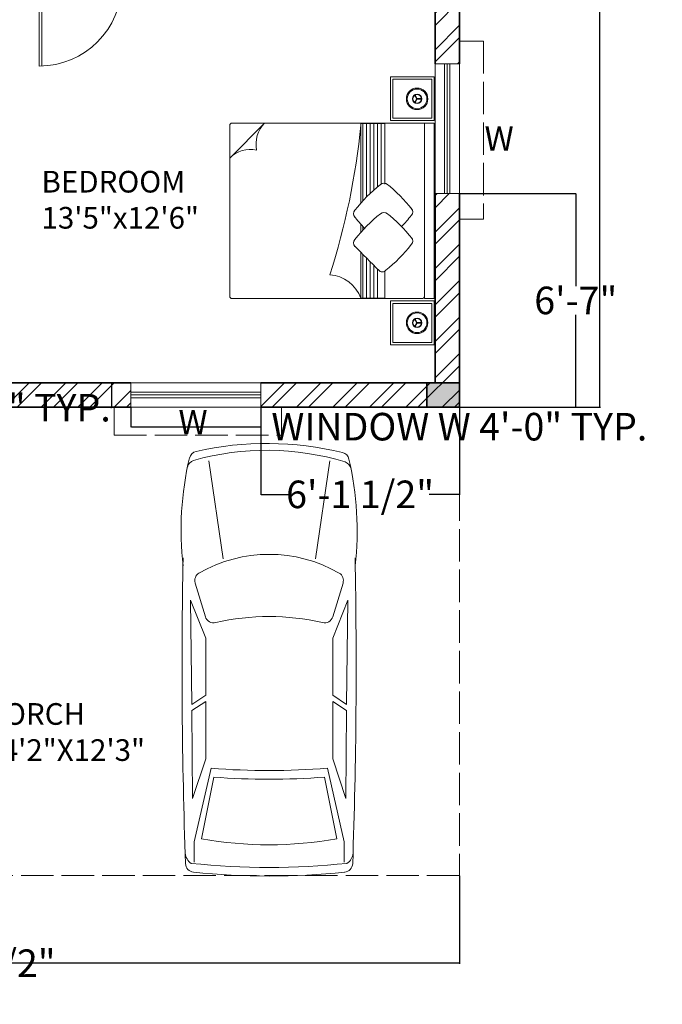
# Model space of a CAD drawing. Units: inches. Extents: x 2379 to 3013, y 1431 to 2110.
# Tile 2 of 10: x 2775 to 3013, y 1431 to 1795. Entities that reach past the tile are written whole.
import ezdxf

# ---------------------------------------------------------------- set-up
doc = ezdxf.new("R2010")
doc.units = ezdxf.units.IN
doc.linetypes.add('ACAD_ISO02W100', pattern=[15, 12, -3])
for name, color, linetype, lineweight in [('00 FURNITURE', 15, 'Continuous', 15), ('A-ANNO-DIMS', 2, 'Continuous', 18), ('A-ANNO-TEXT', 7, 'Continuous', 18), ('A-AREA-IDEN', 7, 'Continuous', 18), ('A-COLS', 7, 'Continuous', 35), ('A-COLS-PATT', 252, 'Continuous', 13), ('A-DOOR', 4, 'Continuous', 18), ('A-ROOF-OVHD', 11, 'ACAD_ISO02W100', 13), ('A-SITE-VEHI', 8, 'Continuous', 13), ('A-WALL-PATT', 8, 'Continuous', 13), ('WALL', 7, 'Continuous', 35), ('WINDOW', 4, 'Continuous', 15)]:
    doc.layers.add(name, color=color, linetype=linetype, lineweight=lineweight)
doc.styles.get("Standard").update_dxf_attribs({"font": 'arial.ttf'})
doc.dimstyles.get("Standard").update_dxf_attribs({"dimtxt": 10.18, "dimasz": 0.18, "dimexe": 0.18, "dimexo": 0.0625, "dimgap": 0.09, "dimtad": 0, "dimtih": 1, "dimtoh": 1, "dimdec": 0, "dimzin": 0, "dimdsep": 46, "dimlunit": 3, "dimtxsty": 'Standard', "dimcen": 0.09, "dimadec": 0, "dimazin": 0, "dimtfac": 1, "dimtdec": 0, "dimtofl": 0, "dimtmove": 0, "dimatfit": 3, "dimfxl": 1, "dimtolj": 1, "dimtzin": 0, "dimarcsym": 0})

# ---------------------------------------------------------------- blocks, each defined once
blk = doc.blocks.new('column')
for p, q in [((2588.21, 2021.79), (2597.21, 2021.79)), ((2588.21, 2009.79), (2588.21, 2021.79)), ((2597.21, 2021.79), (2597.21, 2009.79)), ((2597.21, 2009.79), (2588.21, 2009.79))]:
    blk.add_line(p, q)
blk = doc.blocks.new('DDD')
at = {"layer": '00 FURNITURE'}
for p, q in [((-12579.77, -15859.53), (-12579.77, -15829.05)), ((-12578.77, -15859.53), (-12578.77, -15829.03)), ((-12612.02, -15857.03), (-12612.02, -15862.03)), ((-12611.02, -15857.03), (-12612.02, -15857.03)), ((-12610.52, -15858.03), (-12610.52, -15857.53)), ((-12577.52, -15858.03), (-12577.52, -15857.53)), ((-12577.02, -15857.03), (-12576.02, -15857.03)), ((-12576.02, -15857.03), (-12576.02, -15862.03)), ((-12612.02, -15862.03), (-12611.02, -15862.03)), ((-12610.52, -15861.53), (-12610.52, -15861.03)), ((-12578.77, -15859.53), (-12579.77, -15859.53)), ((-12577.52, -15861.53), (-12577.52, -15861.03)), ((-12576.02, -15862.03), (-12577.02, -15862.03))]:
    blk.add_line(p, q, dxfattribs=at)
for points in [[(-12610.52, -15861.03), (-12610.02, -15861.03, 0.414214), (-12609.52, -15860.53), (-12609.52, -15858.53, 0.414214), (-12610.02, -15858.03), (-12610.52, -15858.03)], [(-12577.52, -15861.03), (-12578.02, -15861.03, -0.414214), (-12578.52, -15860.53), (-12578.52, -15858.53, -0.414214), (-12578.02, -15858.03), (-12577.52, -15858.03)]]:
    blk.add_lwpolyline(points, format="xyb", dxfattribs=at)
for centre, radius, start, end in [((-12578.77, -15859.53), 30.5, 90, 180), ((-12611.02, -15857.53), 0.5, 0, 90), ((-12577.02, -15857.53), 0.5, 90, 180), ((-12611.02, -15861.53), 0.5, 270, 0), ((-12577.02, -15861.53), 0.5, 180, 270)]:
    blk.add_arc(centre, radius, start, end, dxfattribs=at)
blk = doc.blocks.new('RGWTG')
at = {"layer": '00 FURNITURE'}
for p, q in [((578.23, 3473.51), (577.36, 3475.01)), ((578.23, 3473.58), (577.36, 3472.08)), ((578.36, 3473.58), (577.49, 3475.09)), ((578.36, 3473.51), (577.49, 3472)), ((578.29, 3473.62), (580.03, 3473.62)), ((578.29, 3473.47), (580.03, 3473.47)), ((521.93, 3464.58), (509.03, 3451.68)), ((509.03, 3422.63), (509.03, 3463.68)), ((509.93, 3464.58), (566.4, 3464.58)), ((557.53, 3463.84), (557.53, 3464.49)), ((557.53, 3464.49), (566.4, 3464.49)), ((558.2, 3464.49), (558.2, 3435.82)), ((559.57, 3464.49), (559.57, 3437.25)), ((560.94, 3464.49), (560.94, 3438.58)), ((562.3, 3464.49), (562.3, 3439.83)), ((563.67, 3464.49), (563.67, 3440.99)), ((565.04, 3464.49), (565.04, 3442.08)), ((566.4, 3464.58), (580.98, 3464.58)), ((566.4, 3464.49), (566.4, 3442.08)), ((566.4, 3464.49), (566.4, 3463.84)), ((580.98, 3464.58), (580.98, 3416.72)), ((558.2, 3426.48), (558.2, 3425.04)), ((509.03, 3400.68), (509.03, 3422.63)), ((558.2, 3416.13), (558.2, 3399.95)), ((559.57, 3414.75), (559.57, 3399.95)), ((580.98, 3416.72), (580.98, 3400.68)), ((560.94, 3413.39), (560.94, 3399.95)), ((562.3, 3412.04), (562.3, 3399.95)), ((563.67, 3410.72), (563.67, 3399.95)), ((557.53, 3399.95), (557.53, 3400.6)), ((566.4, 3400.6), (566.4, 3399.95)), ((580.08, 3399.78), (509.93, 3399.78)), ((566.4, 3399.95), (557.53, 3399.95)), ((578.23, 3390.78), (577.36, 3392.29)), ((578.23, 3390.86), (577.36, 3389.36)), ((578.36, 3390.86), (577.49, 3392.36)), ((578.36, 3390.78), (577.49, 3389.28)), ((578.29, 3390.9), (580.03, 3390.9)), ((578.29, 3390.74), (580.03, 3390.74))]:
    blk.add_line(p, q, dxfattribs=at)
for points in [[(568.43, 3465.48), (584.63, 3465.48), (584.63, 3481.68), (568.43, 3481.68)], [(569.33, 3466.38), (583.73, 3466.38), (583.73, 3480.78), (569.33, 3480.78)], [(580.98, 3399.78), (584.63, 3399.78), (584.63, 3464.58), (580.98, 3464.58)], [(568.43, 3398.88), (584.63, 3398.88), (584.63, 3382.68), (568.43, 3382.68)], [(569.33, 3397.98), (583.73, 3397.98), (583.73, 3383.58), (569.33, 3383.58)]]:
    blk.add_lwpolyline(points, close=True, dxfattribs=at)
for points in [[(566.52, 3464.49), (557.53, 3464.49), (557.53, 3435.08)], [(557.53, 3427.21), (557.53, 3424.3)], [(557.53, 3416.82), (557.53, 3399.95), (566.4, 3399.95), (566.4, 3409.94)]]:
    blk.add_lwpolyline(points, dxfattribs=at)
for centre, radius in [((578.29, 3473.54), 3.97), ((578.29, 3473.54), 3.63), ((578.29, 3473.54), 1.74), ((578.29, 3473.54), 1.56), ((578.29, 3390.82), 3.97), ((578.29, 3390.82), 3.63), ((578.29, 3390.82), 1.74), ((578.29, 3390.82), 1.56)]:
    blk.add_circle(centre, radius, dxfattribs=at)
for centre, radius, start, end in [((509.93, 3463.68), 0.9, 90, 180), ((529.65, 3456.88), 10.9, 135.0361, 191.9278), ((290.56, 3490.52), 268.3, 342.2214, 354.2925), ((516.73, 3443.97), 10.9, 78.0722, 134.9639), ((598.15, 3399.01), 54.32, 127.931, 142.069), ((566.05, 3440.57), 1.82, 45, 135), ((533.58, 3399.31), 54.32, 37.931, 52.069), ((574.84, 3431.77), 1.82, 315, 45), ((556.59, 3431.11), 1.82, 135, 225), ((597.87, 3463.6), 54.32, 217.931, 224.141), ((598.15, 3388.23), 54.32, 127.931, 142.069), ((566.05, 3429.78), 1.82, 45, 135), ((533.58, 3388.53), 54.32, 37.931, 52.069), ((533.28, 3463.88), 54.32, 316.32, 322.069), ((574.84, 3420.99), 1.82, 315, 45), ((556.59, 3420.33), 1.82, 135, 225), ((765.33, 3619.75), 290.45, 223.6069, 226.2326), ((533.28, 3453.1), 54.32, 307.931, 322.069), ((545.02, 3395.29), 13.35, 20.4224, 85.5825), ((565.44, 3411.05), 1.47, 225.9674, 326.8337), ((509.93, 3400.68), 0.9, 180, 270), ((580.08, 3400.68), 0.9, 270, 0)]:
    blk.add_arc(centre, radius, start, end, dxfattribs=at)
blk = doc.blocks.new('*D15')
at = {"layer": 'A-ANNO-DIMS', "color": 0, "lineweight": -2, "transparency": 16777216}
for p, q in [((2937.69, 2021.61), (2989.73, 2021.61)), ((2989.55, 2021.43), (2989.55, 1841.9)), ((2989.55, 1651.79), (2989.55, 1831.32)), ((2937.69, 1651.61), (2989.73, 1651.61))]:
    blk.add_line(p, q, dxfattribs=at)
at = {"layer": 'A-ANNO-DIMS', "color": 0, "transparency": 16777216}
for points in [[(2989.52, 2021.43), (2989.58, 2021.43), (2989.55, 2021.61)], [(2989.52, 1651.79), (2989.58, 1651.79), (2989.55, 1651.61)]]:
    blk.add_solid(points, dxfattribs=at)
at = {"layer": 'Defpoints', "color": 0, "transparency": 16777216}
for p in [(2937.63, 2021.61), (2937.62, 1651.61), (2989.55, 1651.61)]:
    blk.add_point(p, dxfattribs=at)
at = {"layer": 'A-ANNO-DIMS', "color": 0, "transparency": 16777216, "insert": (2989.55, 1836.61), "char_height": 10.18, "attachment_point": 5}
blk.add_mtext('\\A1;30\'-10"', dxfattribs=at)
blk = doc.blocks.new('WIN-48IN')
for p, q in [((0, 48), (0, 0)), ((9, 48), (0, 48)), ((3.5, 48), (3.5, 0)), ((4.5, 48), (4.5, 0)), ((5.5, 48), (5.5, 0)), ((9, 0), (9, 48)), ((9, 0), (0, 0))]:
    blk.add_line(p, q)
blk = doc.blocks.new('*D22')
at = {"layer": 'A-ANNO-DIMS', "color": 0, "lineweight": -2, "transparency": 16777216}
for p, q in [((2816.22, 1651.55), (2816.22, 1644.23)), ((2864.22, 1651.55), (2864.22, 1644.23)), ((2816.4, 1644.41), (2864.04, 1644.41)), ((2864.22, 1644.41), (2864.4, 1644.41))]:
    blk.add_line(p, q, dxfattribs=at)
at = {"layer": 'A-ANNO-DIMS', "color": 0, "transparency": 16777216}
for points in [[(2816.4, 1644.44), (2816.4, 1644.38), (2816.22, 1644.41)], [(2864.04, 1644.44), (2864.04, 1644.38), (2864.22, 1644.41)]]:
    blk.add_solid(points, dxfattribs=at)
at = {"layer": 'Defpoints', "color": 0, "transparency": 16777216}
for p in [(2816.22, 1651.61), (2864.22, 1651.61), (2864.22, 1644.41)]:
    blk.add_point(p, dxfattribs=at)
at = {"layer": 'A-ANNO-DIMS', "color": 0, "transparency": 16777216, "insert": (2937.59, 1644.41), "char_height": 10.18, "attachment_point": 5}
blk.add_mtext('\\A1;WINDOW W 4\'-0" TYP.', dxfattribs=at)
blk = doc.blocks.new('*D23')
at = {"layer": 'A-ANNO-DIMS', "color": 0, "lineweight": -2, "transparency": 16777216}
for p, q in [((2816.16, 1660.61), (2808.84, 1660.61)), ((2809.02, 1660.43), (2809.02, 1651.79)), ((2816.16, 1651.61), (2808.84, 1651.61)), ((2809.02, 1651.43), (2808.84, 1651.43)), ((2809.02, 1651.61), (2809.02, 1651.43))]:
    blk.add_line(p, q, dxfattribs=at)
at = {"layer": 'A-ANNO-DIMS', "color": 0, "transparency": 16777216}
for points in [[(2808.99, 1660.43), (2809.05, 1660.43), (2809.02, 1660.61)], [(2808.99, 1651.79), (2809.05, 1651.79), (2809.02, 1651.61)]]:
    blk.add_solid(points, dxfattribs=at)
at = {"layer": 'Defpoints', "color": 0, "transparency": 16777216}
for p in [(2816.22, 1660.61), (2809.02, 1651.61), (2816.22, 1651.61)]:
    blk.add_point(p, dxfattribs=at)
at = {"layer": 'A-ANNO-DIMS', "color": 0, "transparency": 16777216, "insert": (2777.72, 1651.43), "char_height": 10.18, "attachment_point": 5}
blk.add_mtext('\\A1;0\'-9" TYP.', dxfattribs=at)
blk = doc.blocks.new('*D53')
at = {"layer": 'A-ANNO-DIMS', "color": 0, "lineweight": -2, "transparency": 16777216}
for p, q in [((2704.97, 1871.8), (2704.97, 1446.07)), ((2735.32, 1871.8), (2735.32, 1446.07)), ((2705.15, 1446.25), (2735.14, 1446.25)), ((2735.32, 1446.25), (2735.5, 1446.25))]:
    blk.add_line(p, q, dxfattribs=at)
at = {"layer": 'A-ANNO-DIMS', "color": 0, "transparency": 16777216}
for points in [[(2705.15, 1446.28), (2705.15, 1446.22), (2704.97, 1446.25)], [(2735.14, 1446.28), (2735.14, 1446.22), (2735.32, 1446.25)]]:
    blk.add_solid(points, dxfattribs=at)
at = {"layer": 'Defpoints', "color": 0, "transparency": 16777216}
for p in [(2704.97, 1871.87), (2735.32, 1871.87), (2735.32, 1446.25)]:
    blk.add_point(p, dxfattribs=at)
at = {"layer": 'A-ANNO-DIMS', "color": 0, "transparency": 16777216, "insert": (2761.07, 1446.25), "char_height": 10.18, "attachment_point": 5}
blk.add_mtext('\\A1;2\'-6 1/2"', dxfattribs=at)
blk = doc.blocks.new('*D62')
at = {"layer": 'A-ANNO-DIMS', "color": 0, "lineweight": -2, "transparency": 16777216}
for p, q in [((2937.69, 1730.48), (2980.8, 1730.48)), ((2980.62, 1730.3), (2980.62, 1696.33)), ((2980.62, 1651.79), (2980.62, 1685.75)), ((2937.69, 1651.61), (2980.8, 1651.61))]:
    blk.add_line(p, q, dxfattribs=at)
at = {"layer": 'A-ANNO-DIMS', "color": 0, "transparency": 16777216}
for points in [[(2980.59, 1730.3), (2980.65, 1730.3), (2980.62, 1730.48)], [(2980.59, 1651.79), (2980.65, 1651.79), (2980.62, 1651.61)]]:
    blk.add_solid(points, dxfattribs=at)
at = {"layer": 'Defpoints', "color": 0, "transparency": 16777216}
for p in [(2937.63, 1730.48), (2980.62, 1730.48), (2937.63, 1651.61)]:
    blk.add_point(p, dxfattribs=at)
at = {"layer": 'A-ANNO-DIMS', "color": 0, "transparency": 16777216, "insert": (2980.62, 1691.04), "char_height": 10.18, "attachment_point": 5}
blk.add_mtext('\\A1;6\'-7"', dxfattribs=at)
blk = doc.blocks.new('*D63')
at = {"layer": 'A-ANNO-DIMS', "color": 0, "lineweight": -2, "transparency": 16777216}
for p, q in [((2864.22, 1651.55), (2864.22, 1619.23)), ((2937.63, 1651.55), (2937.63, 1619.23)), ((2864.4, 1619.41), (2875.41, 1619.41)), ((2937.45, 1619.41), (2926.43, 1619.41))]:
    blk.add_line(p, q, dxfattribs=at)
at = {"layer": 'A-ANNO-DIMS', "color": 0, "transparency": 16777216}
for points in [[(2864.4, 1619.44), (2864.4, 1619.38), (2864.22, 1619.41)], [(2937.45, 1619.44), (2937.45, 1619.38), (2937.63, 1619.41)]]:
    blk.add_solid(points, dxfattribs=at)
at = {"layer": 'Defpoints', "color": 0, "transparency": 16777216}
for p in [(2864.22, 1651.61), (2937.63, 1651.61), (2864.22, 1619.41)]:
    blk.add_point(p, dxfattribs=at)
at = {"layer": 'A-ANNO-DIMS', "color": 0, "transparency": 16777216, "insert": (2900.92, 1619.41), "char_height": 10.18, "attachment_point": 5}
blk.add_mtext('\\A1;6\'-1 1/2"', dxfattribs=at)
blk = doc.blocks.new('*D69')
at = {"layer": 'A-ANNO-DIMS', "color": 0, "lineweight": -2, "transparency": 16777216}
for p, q in [((2539.63, 1478.55), (2539.63, 1446.07)), ((2937.63, 1478.55), (2937.63, 1446.07)), ((2539.81, 1446.25), (2721.06, 1446.25)), ((2937.45, 1446.25), (2756.2, 1446.25))]:
    blk.add_line(p, q, dxfattribs=at)
at = {"layer": 'A-ANNO-DIMS', "color": 0, "transparency": 16777216}
for points in [[(2539.81, 1446.28), (2539.81, 1446.22), (2539.63, 1446.25)], [(2937.45, 1446.28), (2937.45, 1446.22), (2937.63, 1446.25)]]:
    blk.add_solid(points, dxfattribs=at)
at = {"layer": 'Defpoints', "color": 0, "transparency": 16777216}
for p in [(2539.63, 1478.61), (2937.63, 1478.61), (2937.63, 1446.25)]:
    blk.add_point(p, dxfattribs=at)
at = {"layer": 'A-ANNO-DIMS', "color": 0, "transparency": 16777216, "insert": (2738.63, 1446.25), "char_height": 10.18, "attachment_point": 5}
blk.add_mtext('\\A1;33\'-2"', dxfattribs=at)

msp = doc.modelspace()

# ---------------------------------------------------------------- hatches: boundary and pattern name
at = {"layer": 'A-COLS-PATT'}
h = msp.add_hatch(color=256, dxfattribs=at)
h.dxf.hatch_style = 1
h.paths.add_polyline_path([(2937.62, 1660.61), (2925.62, 1660.61), (2925.62, 1651.61), (2937.62, 1651.61)])
h.paths.add_polyline_path([(2481.63, 1809.61), (2478.63, 1809.61), (2478.63, 1811.02), (2469.63, 1811.02), (2469.63, 1802.02), (2478.63, 1802.02), (2478.63, 1805.61), (2481.63, 1805.61)])
h.paths.add_polyline_path([(2481.63, 1811.02), (2478.63, 1811.02), (2478.63, 1809.61), (2481.63, 1809.61)], flags=17)
h.paths.add_polyline_path([(2481.63, 1805.61), (2478.63, 1805.61), (2478.63, 1802.02), (2481.63, 1802.02)], flags=17)
h.paths.add_polyline_path([(2481.63, 1660.61), (2469.63, 1660.61), (2469.63, 1651.61), (2481.63, 1651.61)])
h.paths.add_polyline_path([(2692.07, 1660.61), (2688.63, 1660.61), (2688.63, 1663.61), (2684.63, 1663.61), (2684.63, 1660.61), (2683.07, 1660.61), (2683.07, 1651.61), (2692.07, 1651.61)])
h.paths.add_polyline_path([(2692.07, 1663.61), (2688.63, 1663.61), (2688.63, 1660.61), (2692.07, 1660.61)], flags=17)
h.paths.add_polyline_path([(2684.63, 1663.61), (2683.07, 1663.61), (2683.07, 1660.61), (2684.63, 1660.61)], flags=17)
h.paths.add_polyline_path([(2770.63, 1660.61), (2767.63, 1660.61), (2767.63, 1663.61), (2763.63, 1663.61), (2763.63, 1660.61), (2761.63, 1660.61), (2761.63, 1651.61), (2763.63, 1651.61), (2767.63, 1651.61), (2767.63, 1651.61), (2770.63, 1651.61)])
h.paths.add_polyline_path([(2770.63, 1663.61), (2767.63, 1663.61), (2767.63, 1660.61), (2770.63, 1660.61)], flags=17)
h.paths.add_polyline_path([(2763.63, 1663.61), (2761.63, 1663.61), (2761.63, 1660.61), (2763.63, 1660.61)], flags=17)
h.paths.add_polyline_path([(2937.63, 1813.62), (2928.63, 1813.62), (2928.63, 1810.61), (2925.63, 1810.61), (2925.63, 1806.61), (2928.63, 1806.61), (2928.63, 1804.62), (2937.63, 1804.62)], flags=17)
h.paths.add_polyline_path([(2937.63, 1813.62), (2928.63, 1813.62), (2928.63, 1810.61), (2925.63, 1810.61), (2925.63, 1804.62), (2937.63, 1804.62)], flags=17)
h.paths.add_polyline_path([(2928.63, 1813.62), (2925.63, 1813.62), (2925.63, 1810.61), (2928.63, 1810.61)], flags=0)
h.paths.add_polyline_path([(2937.63, 1863.8), (2928.63, 1863.8), (2928.63, 1862.61), (2925.63, 1862.61), (2925.63, 1858.61), (2928.63, 1858.61), (2928.63, 1854.8), (2937.63, 1854.8)])
h.paths.add_polyline_path([(2928.63, 1863.8), (2925.63, 1863.8), (2925.63, 1862.61), (2928.63, 1862.61)], flags=17)
h.paths.add_polyline_path([(2928.63, 1858.61), (2925.63, 1858.61), (2925.63, 1854.8), (2928.63, 1854.8)], flags=17)
h.paths.add_polyline_path([(2937.63, 2021.61), (2928.63, 2021.61), (2928.63, 2012.61), (2928.63, 2012.61), (2928.63, 2009.61), (2937.63, 2009.61)])
h.paths.add_polyline_path([(2770.27, 2021.61), (2761.27, 2021.61), (2761.27, 2012.61), (2763.63, 2012.61), (2763.63, 2009.61), (2767.63, 2009.61), (2767.63, 2012.61), (2770.27, 2012.61)])
h.paths.add_polyline_path([(2763.63, 2012.61), (2761.27, 2012.61), (2761.27, 2009.61), (2763.63, 2009.61)], flags=17)
h.paths.add_polyline_path([(2770.27, 2012.61), (2767.63, 2012.61), (2767.63, 2009.61), (2770.27, 2009.61)], flags=17)
h.paths.add_polyline_path([(2597.21, 2021.61), (2588.21, 2021.61), (2588.21, 2012.61), (2590.63, 2012.61), (2590.63, 2009.61), (2594.63, 2009.61), (2594.63, 2012.61), (2597.21, 2012.61)])
h.paths.add_polyline_path([(2590.63, 2012.61), (2588.21, 2012.61), (2588.21, 2009.61), (2590.63, 2009.61)], flags=17)
h.paths.add_polyline_path([(2597.21, 2012.61), (2594.63, 2012.61), (2594.63, 2009.61), (2597.21, 2009.61)], flags=17)
at = {"layer": 'A-WALL-PATT'}
h = msp.add_hatch(dxfattribs=at)
h.set_pattern_fill('ANSI32', color=256)
h.paths.add_polyline_path([(2925.63, 1862.61), (2815.63, 1862.61), (2815.63, 1858.61), (2827.63, 1858.61), (2827.63, 1810.61), (2815.63, 1810.61), (2815.63, 1806.61), (2850.78, 1806.61), (2850.78, 1810.61), (2831.63, 1810.61), (2831.63, 1858.61), (2925.63, 1858.61)])
h.paths.add_polyline_path([(2925.63, 1810.61), (2880.78, 1810.61), (2880.78, 1806.61), (2925.63, 1806.61)], flags=17)
h.paths.add_polyline_path([(2633.75, 1660.61), (2594.63, 1660.61), (2481.63, 1660.61), (2481.63, 1651.61), (2588.63, 1651.61), (2588.63, 1570.61), (2624.28, 1570.61), (2624.28, 1574.61), (2592.63, 1574.61), (2592.63, 1651.61), (2633.75, 1651.61)])
h.paths.add_polyline_path([(2594.63, 1809.61), (2481.63, 1809.61), (2481.63, 1805.61), (2594.63, 1805.61)])
h.paths.add_polyline_path([(2594.63, 2012.61), (2597.21, 2012.61), (2597.21, 2021.61), (2588.21, 2021.61), (2588.21, 2012.61), (2590.63, 2012.61), (2590.63, 1845.61), (2594.63, 1845.61)])
h.paths.add_polyline_path([(2767.63, 2012.61), (2770.27, 2012.61), (2770.27, 2021.61), (2761.27, 2021.61), (2761.27, 2012.61), (2763.63, 2012.61), (2763.63, 1928.61), (2691.63, 1928.61), (2643.63, 1928.61), (2643.63, 1924.61), (2691.63, 1924.61), (2763.63, 1924.61), (2763.63, 1858.61), (2779.63, 1858.61), (2779.63, 1862.61), (2767.63, 1862.61)])
h.paths.add_polyline_path([(2613.63, 2012.61), (2613.63, 2021.61), (2597.21, 2021.61), (2597.21, 2012.61)])
h.paths.add_polyline_path([(2508.33, 2012.61), (2508.33, 2021.61), (2478.63, 2021.61), (2478.63, 2012.61)])
h.paths.add_polyline_path([(2556.33, 2021.61), (2556.33, 2012.61), (2588.21, 2012.61), (2588.21, 2021.61)])
h.paths.add_polyline_path([(2659.15, 2012.61), (2659.15, 2021.61), (2643.63, 2021.61), (2643.63, 1958.61), (2661.63, 1958.61), (2661.63, 1962.61), (2647.63, 1962.61), (2647.63, 2012.61)])
h.paths.add_polyline_path([(2714.17, 2012.61), (2714.17, 2021.61), (2683.15, 2021.61), (2683.15, 2012.61), (2691.63, 2012.61), (2691.63, 1958.61), (2695.63, 1958.61), (2695.63, 2012.61)])
h.paths.add_polyline_path([(2738.17, 2021.61), (2738.17, 2012.61), (2761.27, 2012.61), (2761.27, 2021.61)])
h.paths.add_polyline_path([(2820.76, 2012.61), (2820.76, 2021.61), (2770.27, 2021.61), (2770.27, 2012.61)])
h.paths.add_polyline_path([(2868.76, 2021.61), (2868.76, 2012.61), (2928.63, 2012.61), (2928.63, 2021.61)])
h.paths.add_polyline_path([(2928.63, 1962.9), (2937.63, 1962.9), (2937.63, 2009.61), (2928.63, 2009.61)])
h.paths.add_polyline_path([(2937.63, 1914.9), (2928.63, 1914.9), (2928.63, 1863.8), (2937.63, 1863.8)])
h.paths.add_polyline_path([(2928.63, 1846.59), (2937.63, 1846.59), (2937.63, 1854.8), (2928.63, 1854.8)])
h.paths.add_polyline_path([(2937.63, 1822.59), (2928.63, 1822.59), (2928.63, 1813.62), (2937.63, 1813.62)])
h.paths.add_polyline_path([(2928.63, 1778.48), (2937.63, 1778.48), (2937.63, 1813.62), (2928.63, 1813.62), (2928.63, 1810.61), (2925.63, 1810.61), (2925.63, 1806.61), (2928.63, 1806.61)])
h.paths.add_polyline_path([(2816.22, 1651.61), (2816.22, 1660.61), (2767.63, 1660.61), (2767.63, 1806.61), (2779.63, 1806.61), (2779.63, 1810.61), (2763.63, 1810.61), (2763.63, 1660.61), (2688.63, 1660.61), (2688.63, 1810.61), (2684.63, 1810.61), (2684.63, 1660.61), (2669.75, 1660.61), (2669.75, 1651.61), (2763.63, 1651.61), (2763.63, 1574.61), (2672.28, 1574.61), (2672.28, 1570.61), (2767.63, 1570.61), (2767.63, 1651.61)])
h.paths.add_polyline_path([(2864.22, 1660.61), (2864.22, 1651.61), (2937.63, 1651.61), (2937.63, 1730.48), (2928.63, 1730.48), (2928.63, 1660.61)])
h.paths.add_polyline_path([(2469.63, 1975.19), (2478.63, 1975.19), (2478.63, 2009.61), (2469.63, 2009.61)])
h.paths.add_polyline_path([(2478.63, 1927.19), (2469.63, 1927.19), (2469.63, 1811.02), (2478.63, 1811.02)])
h.paths.add_polyline_path([(2469.63, 1758.04), (2478.63, 1758.04), (2478.63, 1802.02), (2469.63, 1802.02)])
h.paths.add_polyline_path([(2478.63, 1710.04), (2469.63, 1710.04), (2469.63, 1660.61), (2478.63, 1660.61)])

# ---------------------------------------------------------------- linework, layer by layer
at = {"layer": 'A-ROOF-OVHD'}
for p, q in [((2937.63, 1786.81), (2946.52, 1786.81)), ((2946.52, 1786.81), (2946.52, 1721.05)), ((2946.52, 1721.05), (2937.63, 1721.05)), ((2810.03, 1651.61), (2810.03, 1641.32)), ((2871.9, 1641.32), (2871.9, 1651.61)), ((2937.63, 1651.61), (2937.63, 1478.61)), ((2810.03, 1641.32), (2871.9, 1641.32)), ((2937.63, 1478.61), (2539.63, 1478.61))]:
    msp.add_line(p, q, dxfattribs=at)
at = {"layer": 'A-SITE-VEHI'}
for p, q in [((2845.04, 1631.8), (2850.37, 1595.55)), ((2889.76, 1631.8), (2884.43, 1595.55)), ((2839.98, 1586.67), (2843.74, 1574.23)), ((2894.61, 1586.67), (2890.85, 1574.23)), ((2838.28, 1580.3), (2843.86, 1566.24)), ((2838.75, 1541.83), (2838.28, 1580.3)), ((2896.38, 1580.3), (2890.8, 1566.24)), ((2895.9, 1541.83), (2896.38, 1580.3)), ((2843.86, 1566.24), (2843.86, 1545.2)), ((2890.8, 1566.24), (2890.8, 1545.2)), ((2843.86, 1545.2), (2838.75, 1541.83)), ((2843.86, 1542.94), (2838.79, 1539.6)), ((2843.86, 1542.94), (2843.86, 1521.69)), ((2890.8, 1545.2), (2895.9, 1541.83)), ((2890.8, 1542.94), (2890.8, 1521.69)), ((2890.8, 1542.94), (2895.87, 1539.6)), ((2839.03, 1507.13), (2838.79, 1539.6)), ((2895.62, 1507.13), (2895.87, 1539.6)), ((2843.86, 1521.69), (2839.03, 1507.13)), ((2890.8, 1521.69), (2895.62, 1507.13)), ((2845.9, 1518.24), (2839.65, 1491.08)), ((2888.84, 1518.25), (2895.09, 1491.08)), ((2842.35, 1492.24), (2846.87, 1514.97)), ((2892.3, 1492.24), (2887.79, 1514.97)), ((2839.65, 1491.08), (2839.65, 1483.62)), ((2895.09, 1491.08), (2895.09, 1483.62))]:
    msp.add_line(p, q, dxfattribs=at)
for centre, radius, start, end in [((2866.43, 1519.06), 119.14, 76.3976, 102.667), ((2950.23, 1606.2), 115.47, 166.6607, 186.5655), ((2841.13, 1632.06), 3.34, 104.3452, 166.6607), ((2866.43, 1536.42), 99.28, 73.0347, 105.8141), ((2893.56, 1631.64), 3.34, 13.1156, 74.5941), ((2840.4, 1628.75), 3.34, 107.8179, 168.3942), ((2894.3, 1628.21), 3.34, 11.3249, 70.8826), ((2784.36, 1606.2), 115.47, 353.4345, 13.1156), ((2867.3, 1545.32), 51.94, 60.0774, 119.9226), ((4908.24, 1555.85), 2073.11, 178.89024, 182.01225), ((826.35, 1555.85), 2073.11, 357.98775, 1.10976), ((2843.04, 1587.6), 3.2, 121.1455, 196.7984), ((2891.55, 1587.6), 3.2, 343.2016, 58.8545), ((2846.8, 1575.15), 3.2, 196.7984, 283.6631), ((2867.3, 1486.06), 88.22, 77.0683, 102.9317), ((2887.79, 1575.15), 3.2, 256.3369, 343.2016), ((2867.29, 1795.67), 278.26, 265.5919, 274.4407), ((2867.3, 1793.86), 279.65, 265.7971, 274.2029), ((2867.3, 1629.7), 139.72, 259.6897, 280.3103), ((2841.16, 1487.27), 4.9, 184.3987, 237.5288), ((2893.43, 1487.27), 4.9, 302.4712, 355.6013), ((2839.75, 1483.18), 3.34, 182.1119, 263.4899), ((2867.3, 1757.49), 275.86, 264.0142, 275.9858), ((2894.84, 1483.18), 3.34, 276.5101, 357.8881), ((2867.3, 1756.41), 277.96, 264.2342, 275.7658)]:
    msp.add_arc(centre, radius, start, end, dxfattribs=at)
at = {"layer": 'WALL'}
for p, q in [((2937.63, 1822.59), (2937.63, 1778.48)), ((2928.63, 1806.61), (2928.63, 1778.48)), ((2928.63, 1730.48), (2928.63, 1660.61)), ((2937.63, 1730.48), (2937.63, 1651.61)), ((2767.63, 1660.61), (2816.22, 1660.61)), ((2864.22, 1660.61), (2928.63, 1660.61)), ((2767.63, 1651.61), (2816.22, 1651.61)), ((2864.22, 1651.61), (2937.63, 1651.61))]:
    msp.add_line(p, q, dxfattribs=at)

# ---------------------------------------------------------------- block references
at = {"layer": '00 FURNITURE'}
msp.add_blockref('RGWTG', (2343.7, -1708.05), dxfattribs=at)
at = {"layer": 'A-COLS', "rotation": 270}
msp.add_blockref('column', (915.84, 4248.82), dxfattribs=at)
at = {"layer": 'A-DOOR', "rotation": 180}
msp.add_blockref('DDD', (-9796.4, -14051.42), dxfattribs=at)
at = {"layer": 'WINDOW'}
for p, rotation in [((2928.63, 1730.48), 359.9999987925818), ((2816.22, 1660.61), 269.9999985709185)]:
    msp.add_blockref('WIN-48IN', p, dxfattribs=dict(at, rotation=rotation))

# ---------------------------------------------------------------- texts
at = {"layer": 'A-ANNO-TEXT', "char_height": 9, "attachment_point": 1}
for insert in [(2946.91, 1755.29), (2833.79, 1650.61)]:
    msp.add_mtext_dynamic_manual_height_columns('W', width=106.8919, gutter_width=12.5, heights=[0], dxfattribs=dict(at, insert=insert))
at = {"layer": 'A-AREA-IDEN', "char_height": 8, "attachment_point": 1}
for s, insert in [('BEDROOM                              13\'5"x12\'6"  ', (2783.19, 1738.89)), ('PORCH\\P14\'2"X12\'3"               ', (2762.44, 1542.3))]:
    msp.add_mtext_dynamic_manual_height_columns(s, width=46.1506, gutter_width=12.5, heights=[0], dxfattribs=dict(at, insert=insert))

# ---------------------------------------------------------------- dimensions: what is measured, and where the dimension line sits
at = {"layer": 'A-ANNO-DIMS'}
for base, p1, p2, angle, override, picture, middle in [((2989.55, 1651.61), (2937.63, 2021.61), (2937.62, 1651.61), 90, {"dimclrd": 0, "dimclre": 0, "dimclrt": 0}, '*D15', (2989.55, 1836.61)), ((2980.62, 1730.48), (2937.63, 1651.61), (2937.63, 1730.48), 90, {"dimdec": 1, "dimlfac": 1, "dimrnd": 0, "dimzin": 1, "dimdsep": 46, "dimlunit": 4, "dimfrac": 2}, '*D62', (2980.62, 1691.04)), ((2864.22, 1619.41), (2937.63, 1651.61), (2864.22, 1651.61), 180, {"dimdec": 1, "dimlfac": 1, "dimrnd": 0, "dimzin": 1, "dimdsep": 46, "dimlunit": 4, "dimfrac": 2}, '*D63', (2900.92, 1619.41))]:
    dim = msp.add_linear_dim(base=base, p1=p1, p2=p2, angle=angle, dimstyle='Standard', override=override, dxfattribs=at)
    dim.commit()
    dim.dimension.update_dxf_attribs({"geometry": picture, "text_midpoint": middle})
for base, p1, p2, picture, middle in [((2735.3226, 1446.2521), (2704.974, 1871.8654), (2735.3226, 1871.8654), '*D53', (2761.0704, 1446.2521)), ((2937.63, 1446.25), (2539.63, 1478.61), (2937.63, 1478.61), '*D69', (2738.63, 1446.25))]:
    dim = msp.add_linear_dim(base=base, p1=p1, p2=p2, dimstyle='Standard', override={"dimdec": 1, "dimlfac": 1, "dimrnd": 0, "dimzin": 1, "dimdsep": 46, "dimlunit": 4, "dimfrac": 2}, dxfattribs=at)
    dim.commit()
    dim.dimension.update_dxf_attribs({"geometry": picture, "text_midpoint": middle})
for base, p1, p2, angle, text, picture, middle in [((2864.22, 1644.41), (2816.22, 1651.61), (2864.22, 1651.61), 360, 'WINDOW W <> TYP.', '*D22', (2937.59, 1644.41)), ((2809.02, 1651.61), (2816.22, 1660.61), (2816.22, 1651.61), 270, '<> TYP.', '*D23', (2777.72, 1651.43))]:
    dim = msp.add_linear_dim(base=base, p1=p1, p2=p2, angle=angle, text=text, dimstyle='Standard', override={"dimdec": 1, "dimlfac": 1, "dimrnd": 0, "dimzin": 1, "dimdsep": 46, "dimlunit": 4, "dimfrac": 2}, dxfattribs=at)
    dim.commit()
    dim.dimension.update_dxf_attribs({"geometry": picture, "text_midpoint": middle})

doc.saveas('drawing.dxf')
